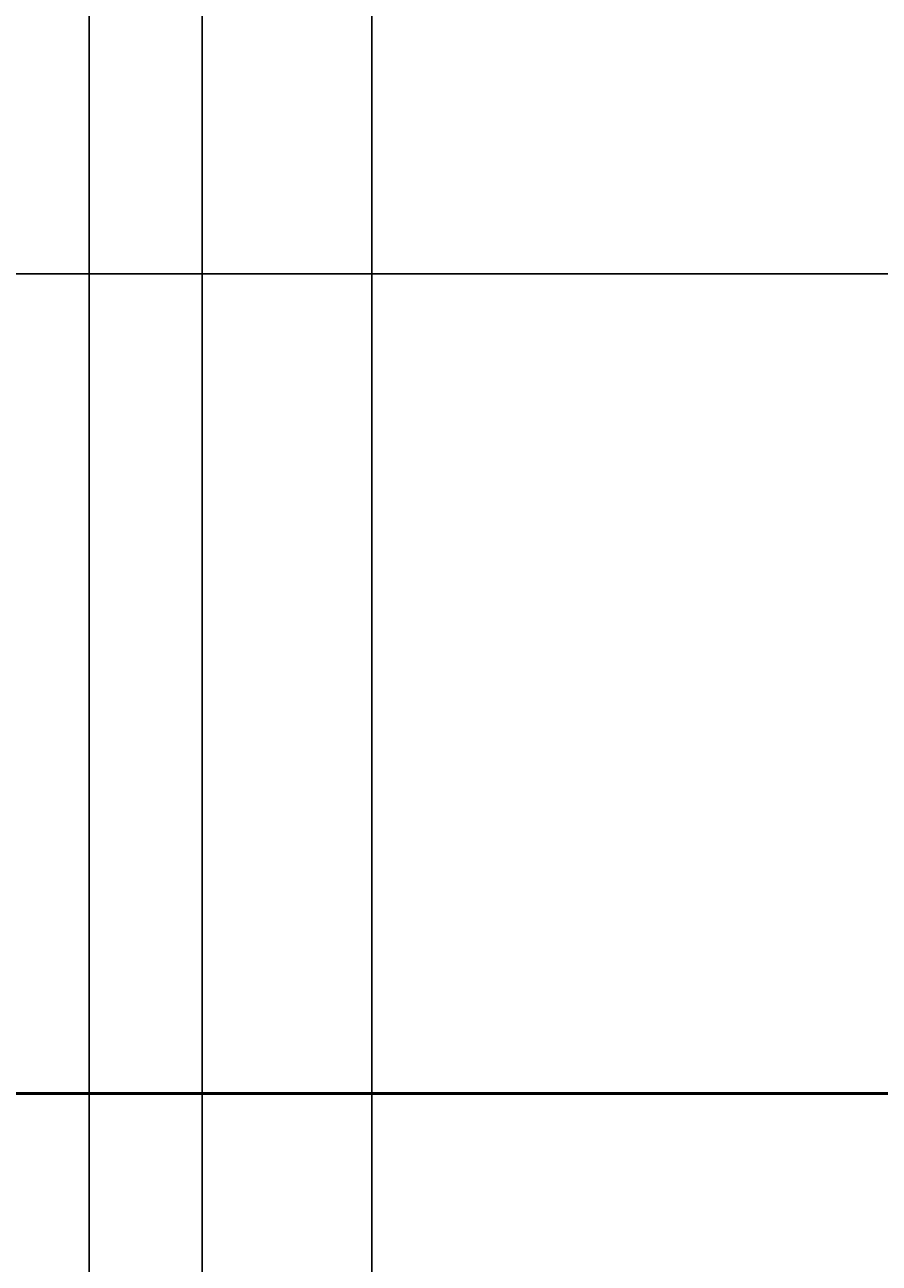
# Model space of a CAD drawing. Units: inches. Extents: x 37 to 824, y -700 to 234.
# Tile 53 of 77: x 204 to 234, y 78 to 122. Entities that reach past the tile are written whole.
import ezdxf

# ---------------------------------------------------------------- set-up
doc = ezdxf.new("R2010")
doc.units = ezdxf.units.IN
doc.header["$MEASUREMENT"] = 0
doc.layers.add('A-ANNO-DIMS', color=2, linetype='Continuous', lineweight=18)
doc.layers.add('A-WALL', color=2, linetype='Continuous', lineweight=50)
doc.styles.get("Standard").update_dxf_attribs({"font": 'arial.ttf'})
doc.dimstyles.get("Standard").update_dxf_attribs({"dimtxt": 0.18, "dimasz": 0.18, "dimexe": 0.18, "dimexo": 0.0625, "dimgap": 0.09, "dimtad": 0, "dimtih": 1, "dimtoh": 1, "dimdec": 1, "dimzin": 0, "dimdsep": 46, "dimlunit": 4, "dimtxsty": 'Standard', "dimcen": 0.09, "dimadec": 0, "dimazin": 0, "dimtfac": 1, "dimtdec": 1, "dimtofl": 0, "dimtmove": 0, "dimatfit": 3, "dimfxl": 1, "dimtolj": 1, "dimtzin": 0, "dimarcsym": 0})

# ---------------------------------------------------------------- blocks, each defined once
blk = doc.blocks.new('*D60')
at = {"layer": 'A-ANNO-DIMS', "color": 0, "lineweight": -2, "ltscale": 0.5, "transparency": 16777216}
for p, q in [((419.015, 113.09), (78.159, 113.09)), ((78.339, 112.91), (78.339, 98.772)), ((78.339, 84.27), (78.339, 98.409)), ((419.015, 84.09), (78.159, 84.09))]:
    blk.add_line(p, q, dxfattribs=at)
at = {"layer": 'A-ANNO-DIMS', "color": 0, "ltscale": 0.5, "transparency": 16777216}
for points in [[(78.309, 112.91), (78.369, 112.91), (78.339, 113.09)], [(78.309, 84.27), (78.369, 84.27), (78.339, 84.09)]]:
    blk.add_solid(points, dxfattribs=at)
at = {"layer": 'Defpoints', "color": 0, "ltscale": 0.5, "transparency": 16777216}
for p in [(78.339, 113.09), (419.077, 113.09), (419.077, 84.09)]:
    blk.add_point(p, dxfattribs=at)
at = {"layer": 'A-ANNO-DIMS', "color": 0, "ltscale": 0.5, "transparency": 16777216, "insert": (78.339, 98.59), "char_height": 0.18, "attachment_point": 5}
blk.add_mtext('\\A1;2\'-5"', dxfattribs=at)
blk = doc.blocks.new('*D72')
at = {"layer": 'A-ANNO-DIMS', "color": 0, "lineweight": -2, "ltscale": 0.5, "transparency": 16777216}
for p, q in [((170.077, 84.153), (170.077, 234.17)), ((170.257, 233.99), (209.804, 233.99)), ((250.01, 233.99), (210.463, 233.99)), ((250.19, 84.153), (250.19, 234.17))]:
    blk.add_line(p, q, dxfattribs=at)
at = {"layer": 'A-ANNO-DIMS', "color": 0, "ltscale": 0.5, "transparency": 16777216}
for points in [[(170.257, 234.02), (170.257, 233.96), (170.077, 233.99)], [(250.01, 234.02), (250.01, 233.96), (250.19, 233.99)]]:
    blk.add_solid(points, dxfattribs=at)
at = {"layer": 'Defpoints', "color": 0, "ltscale": 0.5, "transparency": 16777216}
for p in [(250.19, 233.99), (170.077, 84.09), (250.19, 84.09)]:
    blk.add_point(p, dxfattribs=at)
at = {"layer": 'A-ANNO-DIMS', "color": 0, "ltscale": 0.5, "transparency": 16777216, "insert": (210.133, 233.99), "char_height": 0.18, "attachment_point": 5}
blk.add_mtext('\\A1;6\'-8"', dxfattribs=at)
blk = doc.blocks.new('*D84')
at = {"layer": 'A-ANNO-DIMS', "color": 0, "lineweight": -2, "ltscale": 0.5, "transparency": 16777216}
for p, q in [((170.077, -265.847), (170.077, 234.17)), ((170.257, 233.99), (189.748, 233.99)), ((209.897, 233.99), (190.406, 233.99)), ((210.077, -265.847), (210.077, 234.17))]:
    blk.add_line(p, q, dxfattribs=at)
at = {"layer": 'A-ANNO-DIMS', "color": 0, "ltscale": 0.5, "transparency": 16777216}
for points in [[(170.257, 234.02), (170.257, 233.96), (170.077, 233.99)], [(209.897, 234.02), (209.897, 233.96), (210.077, 233.99)]]:
    blk.add_solid(points, dxfattribs=at)
at = {"layer": 'Defpoints', "color": 0, "ltscale": 0.5, "transparency": 16777216}
for p in [(210.077, 233.99), (170.077, -265.91), (210.077, -265.91)]:
    blk.add_point(p, dxfattribs=at)
at = {"layer": 'A-ANNO-DIMS', "color": 0, "ltscale": 0.5, "transparency": 16777216, "insert": (190.077, 233.99), "char_height": 0.18, "attachment_point": 5}
blk.add_mtext('\\A1;3\'-4"', dxfattribs=at)
blk = doc.blocks.new('*D85')
at = {"layer": 'A-ANNO-DIMS', "color": 0, "lineweight": -2, "ltscale": 0.5, "transparency": 16777216}
for p, q in [((170.077, -356.847), (170.077, 234.17)), ((170.257, 233.99), (187.748, 233.99)), ((205.897, 233.99), (188.406, 233.99)), ((206.077, -356.847), (206.077, 234.17))]:
    blk.add_line(p, q, dxfattribs=at)
at = {"layer": 'A-ANNO-DIMS', "color": 0, "ltscale": 0.5, "transparency": 16777216}
for points in [[(170.257, 234.02), (170.257, 233.96), (170.077, 233.99)], [(205.897, 234.02), (205.897, 233.96), (206.077, 233.99)]]:
    blk.add_solid(points, dxfattribs=at)
at = {"layer": 'Defpoints', "color": 0, "ltscale": 0.5, "transparency": 16777216}
for p in [(206.077, 233.99), (170.077, -356.91), (206.077, -356.91)]:
    blk.add_point(p, dxfattribs=at)
at = {"layer": 'A-ANNO-DIMS', "color": 0, "ltscale": 0.5, "transparency": 16777216, "insert": (188.077, 233.99), "char_height": 0.18, "attachment_point": 5}
blk.add_mtext('\\A1;3\'-0"', dxfattribs=at)
blk = doc.blocks.new('*D86')
at = {"layer": 'A-ANNO-DIMS', "color": 0, "lineweight": -2, "ltscale": 0.5, "transparency": 16777216}
for p, q in [((206.077, -356.847), (206.077, 234.17)), ((206.257, 233.99), (210.678, 233.99)), ((215.897, 233.99), (211.476, 233.99)), ((216.077, -356.847), (216.077, 234.17))]:
    blk.add_line(p, q, dxfattribs=at)
at = {"layer": 'A-ANNO-DIMS', "color": 0, "ltscale": 0.5, "transparency": 16777216}
for points in [[(206.257, 234.02), (206.257, 233.96), (206.077, 233.99)], [(215.897, 234.02), (215.897, 233.96), (216.077, 233.99)]]:
    blk.add_solid(points, dxfattribs=at)
at = {"layer": 'Defpoints', "color": 0, "ltscale": 0.5, "transparency": 16777216}
for p in [(216.077, 233.99), (206.077, -356.91), (216.077, -356.91)]:
    blk.add_point(p, dxfattribs=at)
at = {"layer": 'A-ANNO-DIMS', "color": 0, "ltscale": 0.5, "transparency": 16777216, "insert": (211.077, 233.99), "char_height": 0.18, "attachment_point": 5}
blk.add_mtext('\\A1;0\'-10"', dxfattribs=at)
blk = doc.blocks.new('*D87')
at = {"layer": 'A-ANNO-DIMS', "color": 0, "lineweight": -2, "ltscale": 0.5, "transparency": 16777216}
for p, q in [((216.077, -356.847), (216.077, 234.17)), ((216.257, 233.99), (255.747, 233.99)), ((295.897, 233.99), (256.407, 233.99)), ((296.077, -356.847), (296.077, 234.17))]:
    blk.add_line(p, q, dxfattribs=at)
at = {"layer": 'A-ANNO-DIMS', "color": 0, "ltscale": 0.5, "transparency": 16777216}
for points in [[(216.257, 234.02), (216.257, 233.96), (216.077, 233.99)], [(295.897, 234.02), (295.897, 233.96), (296.077, 233.99)]]:
    blk.add_solid(points, dxfattribs=at)
at = {"layer": 'Defpoints', "color": 0, "ltscale": 0.5, "transparency": 16777216}
for p in [(296.077, 233.99), (216.077, -356.91), (296.077, -356.91)]:
    blk.add_point(p, dxfattribs=at)
at = {"layer": 'A-ANNO-DIMS', "color": 0, "ltscale": 0.5, "transparency": 16777216, "insert": (256.077, 233.99), "char_height": 0.18, "attachment_point": 5}
blk.add_mtext('\\A1;6\'-8"', dxfattribs=at)

msp = doc.modelspace()

# ---------------------------------------------------------------- linework, layer by layer
at = {"layer": 'A-WALL'}
msp.add_line((250.19, 84.09), (170.077, 84.09), dxfattribs=at)

# ---------------------------------------------------------------- dimensions: what is measured, and where the dimension line sits
at = {"layer": 'A-ANNO-DIMS', "ltscale": 0.5}
for base, p1, p2, picture, middle in [((250.19, 233.99), (170.077, 84.09), (250.19, 84.09), '*D72', (210.133, 233.99)), ((210.077, 233.99), (170.077, -265.91), (210.077, -265.91), '*D84', (190.077, 233.99)), ((206.077, 233.99), (170.077, -356.91), (206.077, -356.91), '*D85', (188.077, 233.99)), ((216.077, 233.99), (206.077, -356.91), (216.077, -356.91), '*D86', (211.077, 233.99)), ((296.077, 233.99), (216.077, -356.91), (296.077, -356.91), '*D87', (256.077, 233.99))]:
    dim = msp.add_linear_dim(base=base, p1=p1, p2=p2, dimstyle='Standard', override={"dimdec": 1, "dimlfac": 1, "dimrnd": 0, "dimzin": 1, "dimdsep": 46, "dimlunit": 4, "dimfrac": 2}, dxfattribs=at)
    dim.commit()
    dim.dimension.update_dxf_attribs({"geometry": picture, "text_midpoint": middle})
dim = msp.add_linear_dim(base=(78.339, 113.09), p1=(419.077, 84.09), p2=(419.077, 113.09), angle=90, dimstyle='Standard', override={"dimdec": 1, "dimlfac": 1, "dimrnd": 0, "dimzin": 1, "dimdsep": 46, "dimlunit": 4, "dimfrac": 2}, dxfattribs=at)
dim.commit()
dim.dimension.update_dxf_attribs({"geometry": '*D60', "text_midpoint": (78.339, 98.59)})

doc.saveas('drawing.dxf')
